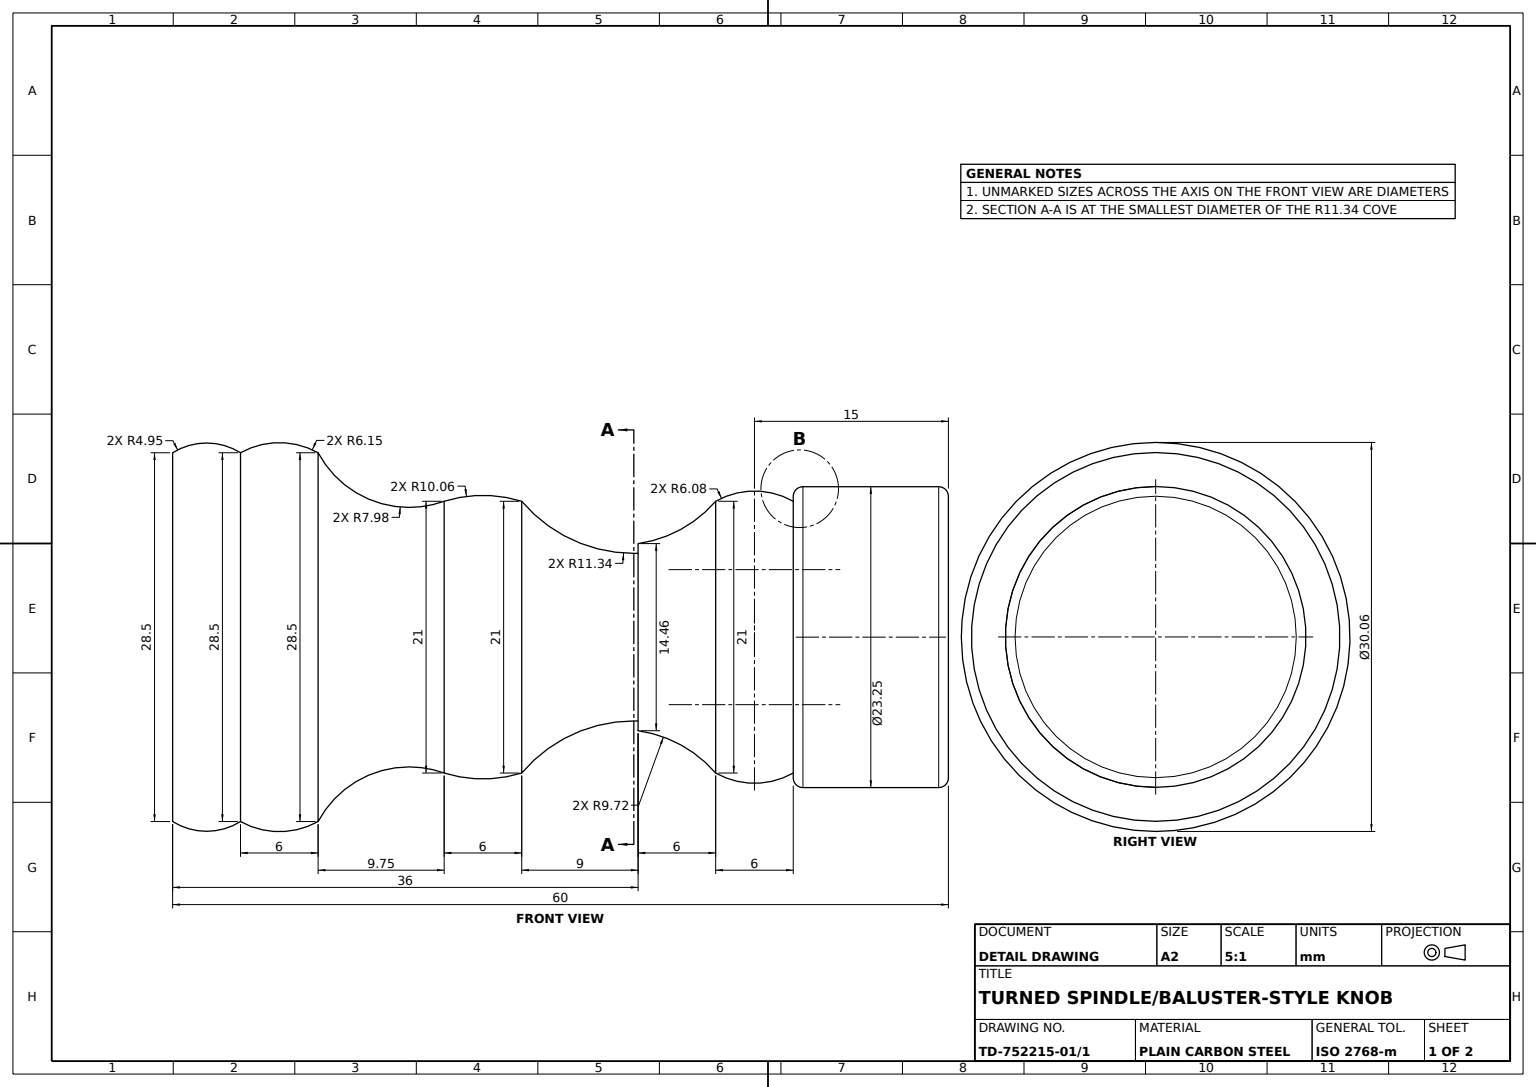
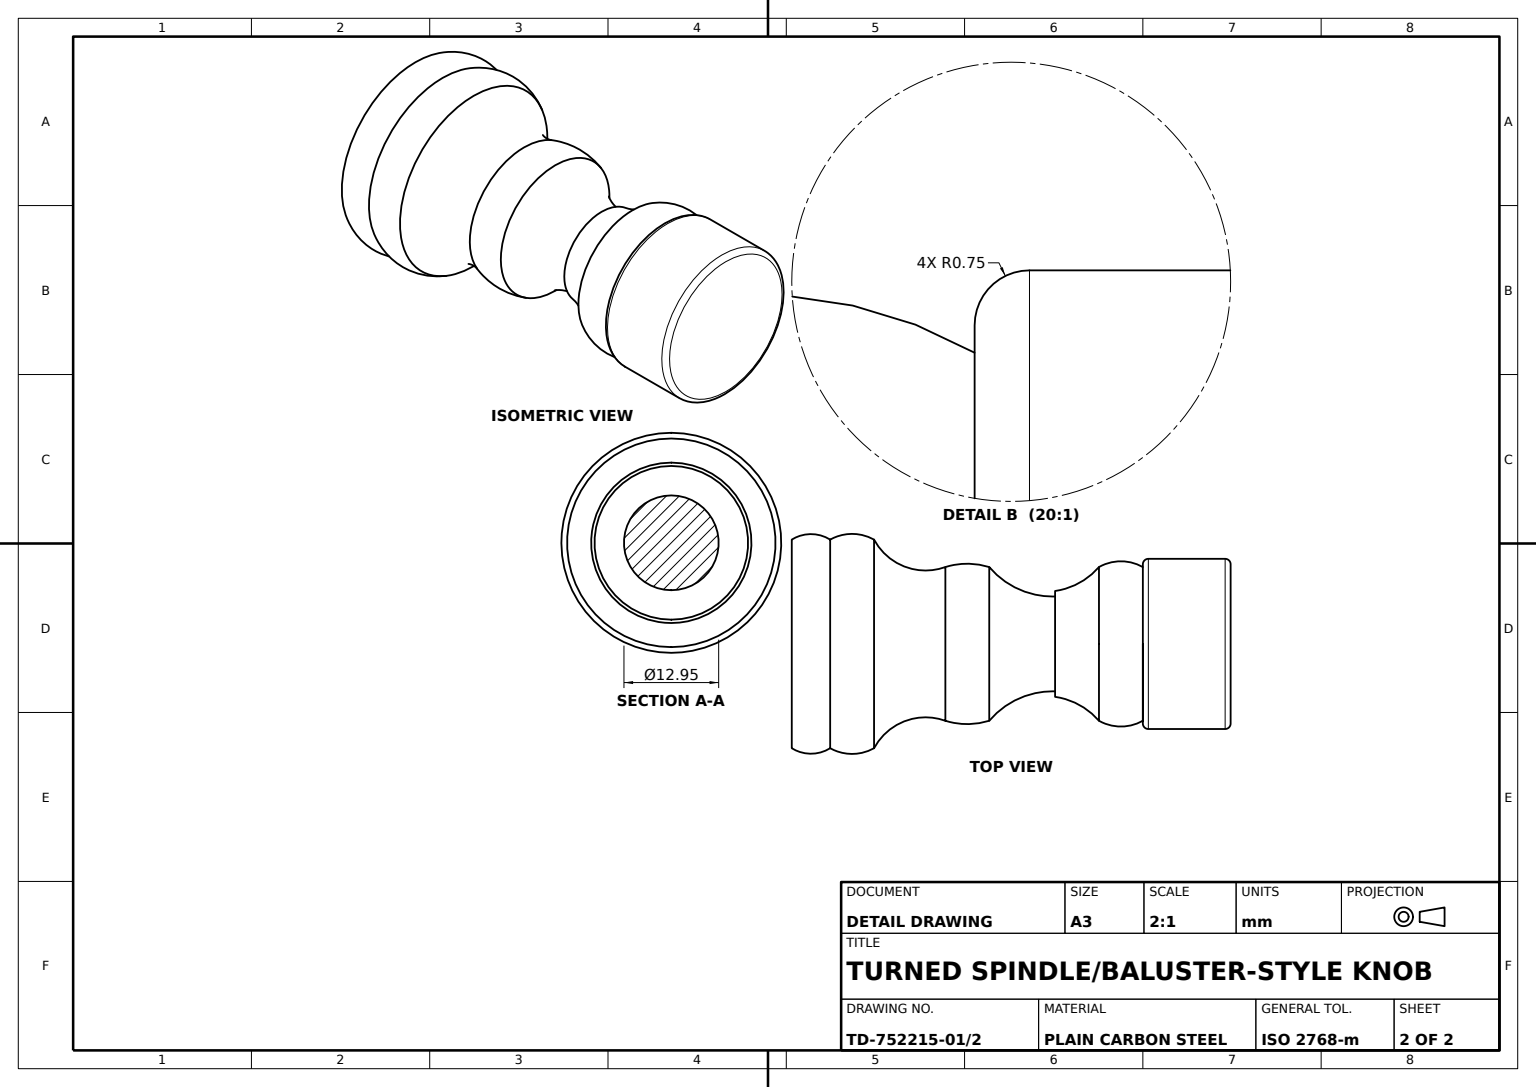
from build123d import *


with BuildPart() as part:
    # Shaft Half-Profile Sketch → Shaft Body Revolve 360° (revolve)
    with BuildSketch(Plane.XY, mode=Mode.PRIVATE) as shaft_body_revolve_360_sk:
        with BuildLine():
            Line((0, 0), (60, 0))
            Line((60, 0), (60, -10.875))
            ThreePointArc((60, -10.875), (59.780330086, -11.405330086), (59.25, -11.625))
            Line((59.25, -11.625), (48.75, -11.625))
            ThreePointArc((48.75, -11.625), (48.219669914, -11.405330086), (48, -10.875))
            Line((48, -10.875), (48, -10.5))
            ThreePointArc((48, -10.5), (45, -11.292422504), (42, -10.5))
            ThreePointArc((42, -10.5), (39.296824458, -8.320367966), (36, -7.23))
            Line((36, -7.23), (36, -6.48))
            ThreePointArc((36, -6.48), (31.040375838, -7.460990683), (27, -10.5))
            ThreePointArc((27, -10.5), (24, -10.957491218), (21, -10.5))
            ThreePointArc((21, -10.5), (15.426129049, -10.557935528), (11.25, -14.25))
            ThreePointArc((11.25, -14.25), (8.25, -15.03134095), (5.25, -14.25))
            ThreePointArc((5.25, -14.25), (2.625, -15.00334955), (0, -14.25))
            Line((0, -14.25), (0, 0))
        make_face()
    revolve(shaft_body_revolve_360_sk.sketch.rotate(Axis((0, 0, 0), (1, 0, 0)), 270), axis=Axis((0, 0, 0), (1, 0, 0)))


solid = part.part
